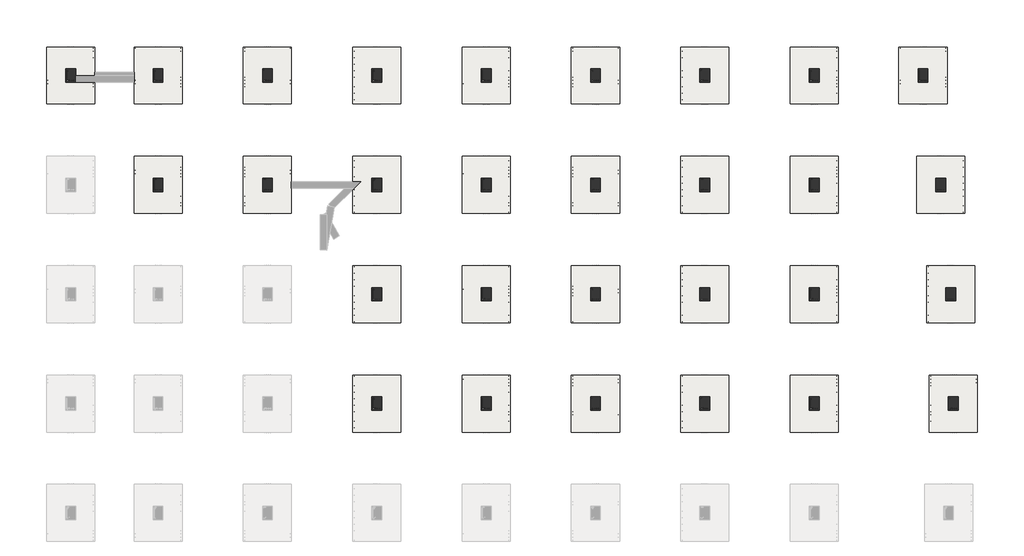
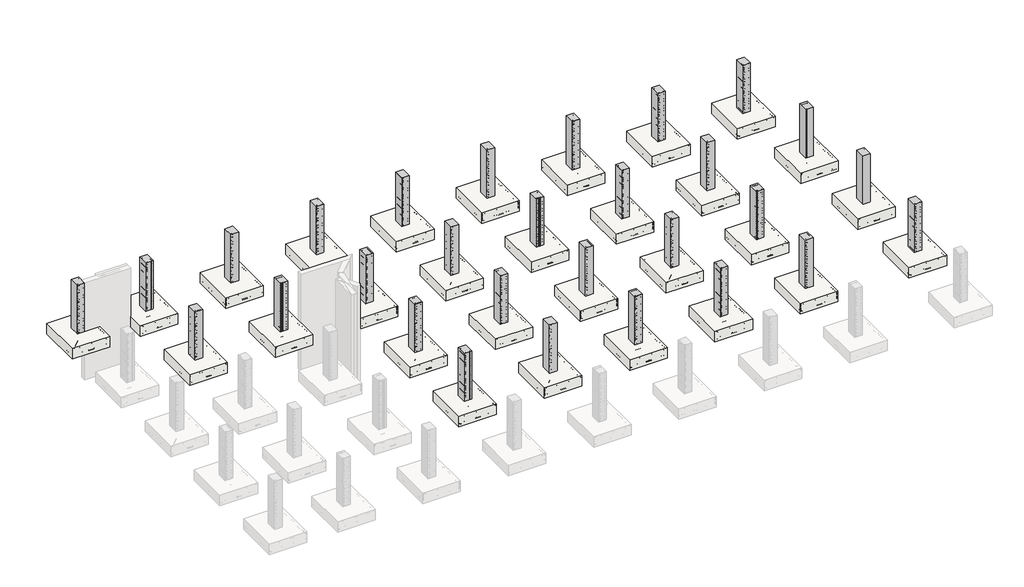
# One storey, part 2 of 33: 29 columns, 29 slabs.
"""IFC4 building model written with IfcOpenShell, lengths in millimetres."""

from ifc_helpers import new_model, si_unit, frame, origin, place, context, project, spatial, polyline, outline, extrude, element, save

model = new_model("IFC4")

# Units and contexts
model_context = context("Model", 3, world=origin())
ifc_project = project(units=[si_unit("LENGTHUNIT", "METRE", prefix="MILLI")], contexts=[model_context])

# Site, building, storey
site = spatial("IfcSite", under=ifc_project)
building = spatial("IfcBuilding", under=site)
storey = spatial("IfcBuildingStorey", under=building, Elevation=-3000.0)

# Columns
placement = place(None, origin())
element("IfcColumn", 1, ObjectType="M_Concrete-Rectangular-Column : 300 x 450mm", at=placement, inside=storey, context=model_context, shape_type="SweptSolid", body=[
    extrude(outline(polyline([(-13414.8142742, 17007.0891866), (-13414.8142742, 16397.4891866), (-13864.8142742, 16397.4891866), (-13864.8142742, 17007.0891866), (-13414.8142742, 17007.0891866)])), frame((0.0, 0.0, -3000.0), z_axis=(0.0, 0.0, 1.0), x_axis=(1.0, 0.0, 0.0)), (0.0, 0.0, 1.0), 3000.0),
])
element("IfcColumn", 2, ObjectType="M_Concrete-Rectangular-Column : 300 x 450mm", at=placement, inside=storey, context=model_context, shape_type="SweptSolid", body=[
    extrude(outline(polyline([(-9414.8142742, 17007.0891866), (-9414.8142742, 16397.4891866), (-9864.8142742, 16397.4891866), (-9864.8142742, 17007.0891866), (-9414.8142742, 17007.0891866)])), frame((0.0, 0.0, -3000.0), z_axis=(0.0, 0.0, 1.0), x_axis=(1.0, 0.0, 0.0)), (0.0, 0.0, 1.0), 3000.0),
])
element("IfcColumn", 3, ObjectType="M_Concrete-Rectangular-Column : 300 x 450mm", at=placement, inside=storey, context=model_context, shape_type="SweptSolid", body=[
    extrude(outline(polyline([(-9414.8142742, 12007.0891866), (-9414.8142742, 11397.4891866), (-9864.8142742, 11397.4891866), (-9864.8142742, 12007.0891866), (-9414.8142742, 12007.0891866)])), frame((0.0, 0.0, -3000.0), z_axis=(0.0, 0.0, 1.0), x_axis=(1.0, 0.0, 0.0)), (0.0, 0.0, 1.0), 3000.0),
])
element("IfcColumn", 4, ObjectType="M_Concrete-Rectangular-Column : 300 x 450mm", at=placement, inside=storey, context=model_context, shape_type="SweptSolid", body=[
    extrude(outline(polyline([(-4414.8142742, 17007.0891866), (-4414.8142742, 16397.4891866), (-4864.8142742, 16397.4891866), (-4864.8142742, 17007.0891866), (-4414.8142742, 17007.0891866)])), frame((0.0, 0.0, -3000.0), z_axis=(0.0, 0.0, 1.0), x_axis=(1.0, 0.0, 0.0)), (0.0, 0.0, 1.0), 3000.0),
])
element("IfcColumn", 5, ObjectType="M_Concrete-Rectangular-Column : 300 x 450mm", at=placement, inside=storey, context=model_context, shape_type="SweptSolid", body=[
    extrude(outline(polyline([(-4414.8142742, 12007.0891866), (-4414.8142742, 11397.4891866), (-4864.8142742, 11397.4891866), (-4864.8142742, 12007.0891866), (-4414.8142742, 12007.0891866)])), frame((0.0, 0.0, -3000.0), z_axis=(0.0, 0.0, 1.0), x_axis=(1.0, 0.0, 0.0)), (0.0, 0.0, 1.0), 3000.0),
])
element("IfcColumn", 6, ObjectType="M_Concrete-Rectangular-Column : 300 x 450mm", at=placement, inside=storey, context=model_context, shape_type="SweptSolid", body=[
    extrude(outline(polyline([(585.1857258, 17007.0891866), (585.1857258, 16397.4891866), (135.1857258, 16397.4891866), (135.1857258, 17007.0891866), (585.1857258, 17007.0891866)])), frame((0.0, 0.0, -3000.0), z_axis=(0.0, 0.0, 1.0), x_axis=(1.0, 0.0, 0.0)), (0.0, 0.0, 1.0), 3000.0),
])
element("IfcColumn", 7, ObjectType="M_Concrete-Rectangular-Column : 300 x 450mm", at=placement, inside=storey, context=model_context, shape_type="SweptSolid", body=[
    extrude(outline(polyline([(585.1857258, 12007.0891866), (585.1857258, 11397.4891866), (135.1857258, 11397.4891866), (135.1857258, 12007.0891866), (585.1857258, 12007.0891866)])), frame((0.0, 0.0, -3000.0), z_axis=(0.0, 0.0, 1.0), x_axis=(1.0, 0.0, 0.0)), (0.0, 0.0, 1.0), 3000.0),
])
element("IfcColumn", 8, ObjectType="M_Concrete-Rectangular-Column : 300 x 450mm", at=placement, inside=storey, context=model_context, shape_type="SweptSolid", body=[
    extrude(outline(polyline([(585.1857258, 7007.0891866), (585.1857258, 6397.4891866), (135.1857258, 6397.4891866), (135.1857258, 7007.0891866), (585.1857258, 7007.0891866)])), frame((0.0, 0.0, -3000.0), z_axis=(0.0, 0.0, 1.0), x_axis=(1.0, 0.0, 0.0)), (0.0, 0.0, 1.0), 3000.0),
])
element("IfcColumn", 9, ObjectType="M_Concrete-Rectangular-Column : 300 x 450mm", at=placement, inside=storey, context=model_context, shape_type="SweptSolid", body=[
    extrude(outline(polyline([(585.1857258, 2007.0891866), (585.1857258, 1397.4891866), (135.1857258, 1397.4891866), (135.1857258, 2007.0891866), (585.1857258, 2007.0891866)])), frame((0.0, 0.0, -3000.0), z_axis=(0.0, 0.0, 1.0), x_axis=(1.0, 0.0, 0.0)), (0.0, 0.0, 1.0), 3000.0),
])
element("IfcColumn", 10, ObjectType="M_Concrete-Rectangular-Column : 300 x 450mm", at=placement, inside=storey, context=model_context, shape_type="SweptSolid", body=[
    extrude(outline(polyline([(5585.1857258, 17007.0891866), (5585.1857258, 16397.4891866), (5135.1857258, 16397.4891866), (5135.1857258, 17007.0891866), (5585.1857258, 17007.0891866)])), frame((0.0, 0.0, -3000.0), z_axis=(0.0, 0.0, 1.0), x_axis=(1.0, 0.0, 0.0)), (0.0, 0.0, 1.0), 3000.0),
])
element("IfcColumn", 11, ObjectType="M_Concrete-Rectangular-Column : 300 x 450mm", at=placement, inside=storey, context=model_context, shape_type="SweptSolid", body=[
    extrude(outline(polyline([(5585.1857258, 12007.0891866), (5585.1857258, 11397.4891866), (5135.1857258, 11397.4891866), (5135.1857258, 12007.0891866), (5585.1857258, 12007.0891866)])), frame((0.0, 0.0, -3000.0), z_axis=(0.0, 0.0, 1.0), x_axis=(1.0, 0.0, 0.0)), (0.0, 0.0, 1.0), 3000.0),
])
element("IfcColumn", 12, ObjectType="M_Concrete-Rectangular-Column : 300 x 450mm", at=placement, inside=storey, context=model_context, shape_type="SweptSolid", body=[
    extrude(outline(polyline([(5585.1857258, 7007.0891866), (5585.1857258, 6397.4891866), (5135.1857258, 6397.4891866), (5135.1857258, 7007.0891866), (5585.1857258, 7007.0891866)])), frame((0.0, 0.0, -3000.0), z_axis=(0.0, 0.0, 1.0), x_axis=(1.0, 0.0, 0.0)), (0.0, 0.0, 1.0), 3000.0),
])
element("IfcColumn", 13, ObjectType="M_Concrete-Rectangular-Column : 300 x 450mm", at=placement, inside=storey, context=model_context, shape_type="SweptSolid", body=[
    extrude(outline(polyline([(5585.1857258, 2007.0891866), (5585.1857258, 1397.4891866), (5135.1857258, 1397.4891866), (5135.1857258, 2007.0891866), (5585.1857258, 2007.0891866)])), frame((0.0, 0.0, -3000.0), z_axis=(0.0, 0.0, 1.0), x_axis=(1.0, 0.0, 0.0)), (0.0, 0.0, 1.0), 3000.0),
])
element("IfcColumn", 14, ObjectType="M_Concrete-Rectangular-Column : 300 x 450mm", at=placement, inside=storey, context=model_context, shape_type="SweptSolid", body=[
    extrude(outline(polyline([(10585.1857258, 17007.0891866), (10585.1857258, 16397.4891866), (10135.1857258, 16397.4891866), (10135.1857258, 17007.0891866), (10585.1857258, 17007.0891866)])), frame((0.0, 0.0, -3000.0), z_axis=(0.0, 0.0, 1.0), x_axis=(1.0, 0.0, 0.0)), (0.0, 0.0, 1.0), 3000.0),
])
element("IfcColumn", 15, ObjectType="M_Concrete-Rectangular-Column : 300 x 450mm", at=placement, inside=storey, context=model_context, shape_type="SweptSolid", body=[
    extrude(outline(polyline([(10585.1857258, 12007.0891866), (10585.1857258, 11397.4891866), (10135.1857258, 11397.4891866), (10135.1857258, 12007.0891866), (10585.1857258, 12007.0891866)])), frame((0.0, 0.0, -3000.0), z_axis=(0.0, 0.0, 1.0), x_axis=(1.0, 0.0, 0.0)), (0.0, 0.0, 1.0), 3000.0),
])
element("IfcColumn", 16, ObjectType="M_Concrete-Rectangular-Column : 300 x 450mm", at=placement, inside=storey, context=model_context, shape_type="SweptSolid", body=[
    extrude(outline(polyline([(10585.1857258, 7007.0891866), (10585.1857258, 6397.4891866), (10135.1857258, 6397.4891866), (10135.1857258, 7007.0891866), (10585.1857258, 7007.0891866)])), frame((0.0, 0.0, -3000.0), z_axis=(0.0, 0.0, 1.0), x_axis=(1.0, 0.0, 0.0)), (0.0, 0.0, 1.0), 3000.0),
])
element("IfcColumn", 17, ObjectType="M_Concrete-Rectangular-Column : 300 x 450mm", at=placement, inside=storey, context=model_context, shape_type="SweptSolid", body=[
    extrude(outline(polyline([(10585.1857258, 2007.0891866), (10585.1857258, 1397.4891866), (10135.1857258, 1397.4891866), (10135.1857258, 2007.0891866), (10585.1857258, 2007.0891866)])), frame((0.0, 0.0, -3000.0), z_axis=(0.0, 0.0, 1.0), x_axis=(1.0, 0.0, 0.0)), (0.0, 0.0, 1.0), 3000.0),
])
element("IfcColumn", 18, ObjectType="M_Concrete-Rectangular-Column : 300 x 450mm", at=placement, inside=storey, context=model_context, shape_type="SweptSolid", body=[
    extrude(outline(polyline([(15585.1857258, 17007.0891866), (15585.1857258, 16397.4891866), (15135.1857258, 16397.4891866), (15135.1857258, 17007.0891866), (15585.1857258, 17007.0891866)])), frame((0.0, 0.0, -3000.0), z_axis=(0.0, 0.0, 1.0), x_axis=(1.0, 0.0, 0.0)), (0.0, 0.0, 1.0), 3000.0),
])
element("IfcColumn", 19, ObjectType="M_Concrete-Rectangular-Column : 300 x 450mm", at=placement, inside=storey, context=model_context, shape_type="SweptSolid", body=[
    extrude(outline(polyline([(15585.1857258, 12007.0891866), (15585.1857258, 11397.4891866), (15135.1857258, 11397.4891866), (15135.1857258, 12007.0891866), (15585.1857258, 12007.0891866)])), frame((0.0, 0.0, -3000.0), z_axis=(0.0, 0.0, 1.0), x_axis=(1.0, 0.0, 0.0)), (0.0, 0.0, 1.0), 3000.0),
])
element("IfcColumn", 20, ObjectType="M_Concrete-Rectangular-Column : 300 x 450mm", at=placement, inside=storey, context=model_context, shape_type="SweptSolid", body=[
    extrude(outline(polyline([(15585.1857258, 7007.0891866), (15585.1857258, 6397.4891866), (15135.1857258, 6397.4891866), (15135.1857258, 7007.0891866), (15585.1857258, 7007.0891866)])), frame((0.0, 0.0, -3000.0), z_axis=(0.0, 0.0, 1.0), x_axis=(1.0, 0.0, 0.0)), (0.0, 0.0, 1.0), 3000.0),
])
element("IfcColumn", 21, ObjectType="M_Concrete-Rectangular-Column : 300 x 450mm", at=placement, inside=storey, context=model_context, shape_type="SweptSolid", body=[
    extrude(outline(polyline([(15585.1857258, 2007.0891866), (15585.1857258, 1397.4891866), (15135.1857258, 1397.4891866), (15135.1857258, 2007.0891866), (15585.1857258, 2007.0891866)])), frame((0.0, 0.0, -3000.0), z_axis=(0.0, 0.0, 1.0), x_axis=(1.0, 0.0, 0.0)), (0.0, 0.0, 1.0), 3000.0),
])
element("IfcColumn", 22, ObjectType="M_Concrete-Rectangular-Column : 300 x 450mm", at=placement, inside=storey, context=model_context, shape_type="SweptSolid", body=[
    extrude(outline(polyline([(20585.1857258, 17007.0891866), (20585.1857258, 16397.4891866), (20135.1857258, 16397.4891866), (20135.1857258, 17007.0891866), (20585.1857258, 17007.0891866)])), frame((0.0, 0.0, -3000.0), z_axis=(0.0, 0.0, 1.0), x_axis=(1.0, 0.0, 0.0)), (0.0, 0.0, 1.0), 3000.0),
])
element("IfcColumn", 23, ObjectType="M_Concrete-Rectangular-Column : 300 x 450mm", at=placement, inside=storey, context=model_context, shape_type="SweptSolid", body=[
    extrude(outline(polyline([(20585.1857258, 12007.0891866), (20585.1857258, 11397.4891866), (20135.1857258, 11397.4891866), (20135.1857258, 12007.0891866), (20585.1857258, 12007.0891866)])), frame((0.0, 0.0, -3000.0), z_axis=(0.0, 0.0, 1.0), x_axis=(1.0, 0.0, 0.0)), (0.0, 0.0, 1.0), 3000.0),
])
element("IfcColumn", 24, ObjectType="M_Concrete-Rectangular-Column : 300 x 450mm", at=placement, inside=storey, context=model_context, shape_type="SweptSolid", body=[
    extrude(outline(polyline([(20585.1857258, 7007.0891866), (20585.1857258, 6397.4891866), (20135.1857258, 6397.4891866), (20135.1857258, 7007.0891866), (20585.1857258, 7007.0891866)])), frame((0.0, 0.0, -3000.0), z_axis=(0.0, 0.0, 1.0), x_axis=(1.0, 0.0, 0.0)), (0.0, 0.0, 1.0), 3000.0),
])
element("IfcColumn", 25, ObjectType="M_Concrete-Rectangular-Column : 300 x 450mm", at=placement, inside=storey, context=model_context, shape_type="SweptSolid", body=[
    extrude(outline(polyline([(20585.1857258, 2007.0891866), (20585.1857258, 1397.4891866), (20135.1857258, 1397.4891866), (20135.1857258, 2007.0891866), (20585.1857258, 2007.0891866)])), frame((0.0, 0.0, -3000.0), z_axis=(0.0, 0.0, 1.0), x_axis=(1.0, 0.0, 0.0)), (0.0, 0.0, 1.0), 3000.0),
])
element("IfcColumn", 26, ObjectType="M_Concrete-Rectangular-Column : 300 x 450mm", at=placement, inside=storey, context=model_context, shape_type="SweptSolid", body=[
    extrude(outline(polyline([(25564.5332373, 17007.0891866), (25564.5332373, 16397.4891866), (25114.5332373, 16397.4891866), (25114.5332373, 17007.0891866), (25564.5332373, 17007.0891866)])), frame((0.0, 0.0, -3000.0), z_axis=(0.0, 0.0, 1.0), x_axis=(1.0, 0.0, 0.0)), (0.0, 0.0, 1.0), 3000.0),
])
element("IfcColumn", 27, ObjectType="M_Concrete-Rectangular-Column : 300 x 450mm", at=placement, inside=storey, context=model_context, shape_type="SweptSolid", body=[
    extrude(outline(polyline([(26372.9223959, 12007.0891866), (26372.9223959, 11397.4891866), (25922.9223959, 11397.4891866), (25922.9223959, 12007.0891866), (26372.9223959, 12007.0891866)])), frame((0.0, 0.0, -3000.0), z_axis=(0.0, 0.0, 1.0), x_axis=(1.0, 0.0, 0.0)), (0.0, 0.0, 1.0), 3000.0),
])
element("IfcColumn", 28, ObjectType="M_Concrete-Rectangular-Column : 300 x 450mm", at=placement, inside=storey, context=model_context, shape_type="SweptSolid", body=[
    extrude(outline(polyline([(26833.3282195, 7007.0891866), (26833.3282195, 6397.4891866), (26383.3282195, 6397.4891866), (26383.3282195, 7007.0891866), (26833.3282195, 7007.0891866)])), frame((0.0, 0.0, -3000.0), z_axis=(0.0, 0.0, 1.0), x_axis=(1.0, 0.0, 0.0)), (0.0, 0.0, 1.0), 3000.0),
])
element("IfcColumn", 29, ObjectType="M_Concrete-Rectangular-Column : 300 x 450mm", at=placement, inside=storey, context=model_context, shape_type="SweptSolid", body=[
    extrude(outline(polyline([(26952.2756413, 2007.0891866), (26952.2756413, 1397.4891866), (26502.2756413, 1397.4891866), (26502.2756413, 2007.0891866), (26952.2756413, 2007.0891866)])), frame((0.0, 0.0, -3000.0), z_axis=(0.0, 0.0, 1.0), x_axis=(1.0, 0.0, 0.0)), (0.0, 0.0, 1.0), 3000.0),
])

# Slabs
element("IfcSlab", 30, ObjectType="M_Footing-Rectangular : 650X2200X2600", at=placement, inside=storey, context=model_context, shape_type="SweptSolid", body=[
    extrude(outline(polyline([(-12539.8142742, 18002.2891866), (-12539.8142742, 15402.2891866), (-14739.8142742, 15402.2891866), (-14739.8142742, 18002.2891866), (-12539.8142742, 18002.2891866)])), frame((0.0, 0.0, -3650.0), z_axis=(0.0, 0.0, 1.0), x_axis=(1.0, 0.0, 0.0)), (0.0, 0.0, 1.0), 650.0),
])
element("IfcSlab", 31, ObjectType="M_Footing-Rectangular : 650X2200X2600", at=placement, inside=storey, context=model_context, shape_type="SweptSolid", body=[
    extrude(outline(polyline([(-8539.8142742, 18002.2891866), (-8539.8142742, 15402.2891866), (-10739.8142742, 15402.2891866), (-10739.8142742, 18002.2891866), (-8539.8142742, 18002.2891866)])), frame((0.0, 0.0, -3650.0), z_axis=(0.0, 0.0, 1.0), x_axis=(1.0, 0.0, 0.0)), (0.0, 0.0, 1.0), 650.0),
])
element("IfcSlab", 32, ObjectType="M_Footing-Rectangular : 650X2200X2600", at=placement, inside=storey, context=model_context, shape_type="SweptSolid", body=[
    extrude(outline(polyline([(-8539.8142742, 13002.2891866), (-8539.8142742, 10402.2891866), (-10739.8142742, 10402.2891866), (-10739.8142742, 13002.2891866), (-8539.8142742, 13002.2891866)])), frame((0.0, 0.0, -3650.0), z_axis=(0.0, 0.0, 1.0), x_axis=(1.0, 0.0, 0.0)), (0.0, 0.0, 1.0), 650.0),
])
element("IfcSlab", 33, ObjectType="M_Footing-Rectangular : 650X2200X2600", at=placement, inside=storey, context=model_context, shape_type="SweptSolid", body=[
    extrude(outline(polyline([(-3539.8142742, 18002.2891866), (-3539.8142742, 15402.2891866), (-5739.8142742, 15402.2891866), (-5739.8142742, 18002.2891866), (-3539.8142742, 18002.2891866)])), frame((0.0, 0.0, -3650.0), z_axis=(0.0, 0.0, 1.0), x_axis=(1.0, 0.0, 0.0)), (0.0, 0.0, 1.0), 650.0),
])
element("IfcSlab", 34, ObjectType="M_Footing-Rectangular : 650X2200X2600", at=placement, inside=storey, context=model_context, shape_type="SweptSolid", body=[
    extrude(outline(polyline([(-3539.8142742, 13002.2891866), (-3539.8142742, 10402.2891866), (-5739.8142742, 10402.2891866), (-5739.8142742, 13002.2891866), (-3539.8142742, 13002.2891866)])), frame((0.0, 0.0, -3650.0), z_axis=(0.0, 0.0, 1.0), x_axis=(1.0, 0.0, 0.0)), (0.0, 0.0, 1.0), 650.0),
])
element("IfcSlab", 35, ObjectType="M_Footing-Rectangular : 650X2200X2600", at=placement, inside=storey, context=model_context, shape_type="SweptSolid", body=[
    extrude(outline(polyline([(1460.1857258, 18002.2891866), (1460.1857258, 15402.2891866), (-739.8142742, 15402.2891866), (-739.8142742, 18002.2891866), (1460.1857258, 18002.2891866)])), frame((0.0, 0.0, -3650.0), z_axis=(0.0, 0.0, 1.0), x_axis=(1.0, 0.0, 0.0)), (0.0, 0.0, 1.0), 650.0),
])
element("IfcSlab", 36, ObjectType="M_Footing-Rectangular : 650X2200X2600", at=placement, inside=storey, context=model_context, shape_type="SweptSolid", body=[
    extrude(outline(polyline([(1460.1857258, 13002.2891866), (1460.1857258, 10402.2891866), (-739.8142742, 10402.2891866), (-739.8142742, 13002.2891866), (1460.1857258, 13002.2891866)])), frame((0.0, 0.0, -3650.0), z_axis=(0.0, 0.0, 1.0), x_axis=(1.0, 0.0, 0.0)), (0.0, 0.0, 1.0), 650.0),
])
element("IfcSlab", 37, ObjectType="M_Footing-Rectangular : 650X2200X2600", at=placement, inside=storey, context=model_context, shape_type="SweptSolid", body=[
    extrude(outline(polyline([(1460.1857258, 8002.2891866), (1460.1857258, 5402.2891866), (-739.8142742, 5402.2891866), (-739.8142742, 8002.2891866), (1460.1857258, 8002.2891866)])), frame((0.0, 0.0, -3650.0), z_axis=(0.0, 0.0, 1.0), x_axis=(1.0, 0.0, 0.0)), (0.0, 0.0, 1.0), 650.0),
])
element("IfcSlab", 38, ObjectType="M_Footing-Rectangular : 650X2200X2600", at=placement, inside=storey, context=model_context, shape_type="SweptSolid", body=[
    extrude(outline(polyline([(1460.1857258, 3002.2891866), (1460.1857258, 402.2891866), (-739.8142742, 402.2891866), (-739.8142742, 3002.2891866), (1460.1857258, 3002.2891866)])), frame((0.0, 0.0, -3650.0), z_axis=(0.0, 0.0, 1.0), x_axis=(1.0, 0.0, 0.0)), (0.0, 0.0, 1.0), 650.0),
])
element("IfcSlab", 39, ObjectType="M_Footing-Rectangular : 650X2200X2600", at=placement, inside=storey, context=model_context, shape_type="SweptSolid", body=[
    extrude(outline(polyline([(6460.1857258, 18002.2891866), (6460.1857258, 15402.2891866), (4260.1857258, 15402.2891866), (4260.1857258, 18002.2891866), (6460.1857258, 18002.2891866)])), frame((0.0, 0.0, -3650.0), z_axis=(0.0, 0.0, 1.0), x_axis=(1.0, 0.0, 0.0)), (0.0, 0.0, 1.0), 650.0),
])
element("IfcSlab", 40, ObjectType="M_Footing-Rectangular : 650X2200X2600", at=placement, inside=storey, context=model_context, shape_type="SweptSolid", body=[
    extrude(outline(polyline([(6460.1857258, 13002.2891866), (6460.1857258, 10402.2891866), (4260.1857258, 10402.2891866), (4260.1857258, 13002.2891866), (6460.1857258, 13002.2891866)])), frame((0.0, 0.0, -3650.0), z_axis=(0.0, 0.0, 1.0), x_axis=(1.0, 0.0, 0.0)), (0.0, 0.0, 1.0), 650.0),
])
element("IfcSlab", 41, ObjectType="M_Footing-Rectangular : 650X2200X2600", at=placement, inside=storey, context=model_context, shape_type="SweptSolid", body=[
    extrude(outline(polyline([(6460.1857258, 8002.2891866), (6460.1857258, 5402.2891866), (4260.1857258, 5402.2891866), (4260.1857258, 8002.2891866), (6460.1857258, 8002.2891866)])), frame((0.0, 0.0, -3650.0), z_axis=(0.0, 0.0, 1.0), x_axis=(1.0, 0.0, 0.0)), (0.0, 0.0, 1.0), 650.0),
])
element("IfcSlab", 42, ObjectType="M_Footing-Rectangular : 650X2200X2600", at=placement, inside=storey, context=model_context, shape_type="SweptSolid", body=[
    extrude(outline(polyline([(6460.1857258, 3002.2891866), (6460.1857258, 402.2891866), (4260.1857258, 402.2891866), (4260.1857258, 3002.2891866), (6460.1857258, 3002.2891866)])), frame((0.0, 0.0, -3650.0), z_axis=(0.0, 0.0, 1.0), x_axis=(1.0, 0.0, 0.0)), (0.0, 0.0, 1.0), 650.0),
])
element("IfcSlab", 43, ObjectType="M_Footing-Rectangular : 650X2200X2600", at=placement, inside=storey, context=model_context, shape_type="SweptSolid", body=[
    extrude(outline(polyline([(11460.1857258, 18002.2891866), (11460.1857258, 15402.2891866), (9260.1857258, 15402.2891866), (9260.1857258, 18002.2891866), (11460.1857258, 18002.2891866)])), frame((0.0, 0.0, -3650.0), z_axis=(0.0, 0.0, 1.0), x_axis=(1.0, 0.0, 0.0)), (0.0, 0.0, 1.0), 650.0),
])
element("IfcSlab", 44, ObjectType="M_Footing-Rectangular : 650X2200X2600", at=placement, inside=storey, context=model_context, shape_type="SweptSolid", body=[
    extrude(outline(polyline([(11460.1857258, 13002.2891866), (11460.1857258, 10402.2891866), (9260.1857258, 10402.2891866), (9260.1857258, 13002.2891866), (11460.1857258, 13002.2891866)])), frame((0.0, 0.0, -3650.0), z_axis=(0.0, 0.0, 1.0), x_axis=(1.0, 0.0, 0.0)), (0.0, 0.0, 1.0), 650.0),
])
element("IfcSlab", 45, ObjectType="M_Footing-Rectangular : 650X2200X2600", at=placement, inside=storey, context=model_context, shape_type="SweptSolid", body=[
    extrude(outline(polyline([(11460.1857258, 8002.2891866), (11460.1857258, 5402.2891866), (9260.1857258, 5402.2891866), (9260.1857258, 8002.2891866), (11460.1857258, 8002.2891866)])), frame((0.0, 0.0, -3650.0), z_axis=(0.0, 0.0, 1.0), x_axis=(1.0, 0.0, 0.0)), (0.0, 0.0, 1.0), 650.0),
])
element("IfcSlab", 46, ObjectType="M_Footing-Rectangular : 650X2200X2600", at=placement, inside=storey, context=model_context, shape_type="SweptSolid", body=[
    extrude(outline(polyline([(11460.1857258, 3002.2891866), (11460.1857258, 402.2891866), (9260.1857258, 402.2891866), (9260.1857258, 3002.2891866), (11460.1857258, 3002.2891866)])), frame((0.0, 0.0, -3650.0), z_axis=(0.0, 0.0, 1.0), x_axis=(1.0, 0.0, 0.0)), (0.0, 0.0, 1.0), 650.0),
])
element("IfcSlab", 47, ObjectType="M_Footing-Rectangular : 650X2200X2600", at=placement, inside=storey, context=model_context, shape_type="SweptSolid", body=[
    extrude(outline(polyline([(16460.1857258, 18002.2891866), (16460.1857258, 15402.2891866), (14260.1857258, 15402.2891866), (14260.1857258, 18002.2891866), (16460.1857258, 18002.2891866)])), frame((0.0, 0.0, -3650.0), z_axis=(0.0, 0.0, 1.0), x_axis=(1.0, 0.0, 0.0)), (0.0, 0.0, 1.0), 650.0),
])
element("IfcSlab", 48, ObjectType="M_Footing-Rectangular : 650X2200X2600", at=placement, inside=storey, context=model_context, shape_type="SweptSolid", body=[
    extrude(outline(polyline([(16460.1857258, 13002.2891866), (16460.1857258, 10402.2891866), (14260.1857258, 10402.2891866), (14260.1857258, 13002.2891866), (16460.1857258, 13002.2891866)])), frame((0.0, 0.0, -3650.0), z_axis=(0.0, 0.0, 1.0), x_axis=(1.0, 0.0, 0.0)), (0.0, 0.0, 1.0), 650.0),
])
element("IfcSlab", 49, ObjectType="M_Footing-Rectangular : 650X2200X2600", at=placement, inside=storey, context=model_context, shape_type="SweptSolid", body=[
    extrude(outline(polyline([(16460.1857258, 8002.2891866), (16460.1857258, 5402.2891866), (14260.1857258, 5402.2891866), (14260.1857258, 8002.2891866), (16460.1857258, 8002.2891866)])), frame((0.0, 0.0, -3650.0), z_axis=(0.0, 0.0, 1.0), x_axis=(1.0, 0.0, 0.0)), (0.0, 0.0, 1.0), 650.0),
])
element("IfcSlab", 50, ObjectType="M_Footing-Rectangular : 650X2200X2600", at=placement, inside=storey, context=model_context, shape_type="SweptSolid", body=[
    extrude(outline(polyline([(16460.1857258, 3002.2891866), (16460.1857258, 402.2891866), (14260.1857258, 402.2891866), (14260.1857258, 3002.2891866), (16460.1857258, 3002.2891866)])), frame((0.0, 0.0, -3650.0), z_axis=(0.0, 0.0, 1.0), x_axis=(1.0, 0.0, 0.0)), (0.0, 0.0, 1.0), 650.0),
])
element("IfcSlab", 51, ObjectType="M_Footing-Rectangular : 650X2200X2600", at=placement, inside=storey, context=model_context, shape_type="SweptSolid", body=[
    extrude(outline(polyline([(21460.1857258, 18002.2891866), (21460.1857258, 15402.2891866), (19260.1857258, 15402.2891866), (19260.1857258, 18002.2891866), (21460.1857258, 18002.2891866)])), frame((0.0, 0.0, -3650.0), z_axis=(0.0, 0.0, 1.0), x_axis=(1.0, 0.0, 0.0)), (0.0, 0.0, 1.0), 650.0),
])
element("IfcSlab", 52, ObjectType="M_Footing-Rectangular : 650X2200X2600", at=placement, inside=storey, context=model_context, shape_type="SweptSolid", body=[
    extrude(outline(polyline([(21460.1857258, 13002.2891866), (21460.1857258, 10402.2891866), (19260.1857258, 10402.2891866), (19260.1857258, 13002.2891866), (21460.1857258, 13002.2891866)])), frame((0.0, 0.0, -3650.0), z_axis=(0.0, 0.0, 1.0), x_axis=(1.0, 0.0, 0.0)), (0.0, 0.0, 1.0), 650.0),
])
element("IfcSlab", 53, ObjectType="M_Footing-Rectangular : 650X2200X2600", at=placement, inside=storey, context=model_context, shape_type="SweptSolid", body=[
    extrude(outline(polyline([(21460.1857258, 8002.2891866), (21460.1857258, 5402.2891866), (19260.1857258, 5402.2891866), (19260.1857258, 8002.2891866), (21460.1857258, 8002.2891866)])), frame((0.0, 0.0, -3650.0), z_axis=(0.0, 0.0, 1.0), x_axis=(1.0, 0.0, 0.0)), (0.0, 0.0, 1.0), 650.0),
])
element("IfcSlab", 54, ObjectType="M_Footing-Rectangular : 650X2200X2600", at=placement, inside=storey, context=model_context, shape_type="SweptSolid", body=[
    extrude(outline(polyline([(21460.1857258, 3002.2891866), (21460.1857258, 402.2891866), (19260.1857258, 402.2891866), (19260.1857258, 3002.2891866), (21460.1857258, 3002.2891866)])), frame((0.0, 0.0, -3650.0), z_axis=(0.0, 0.0, 1.0), x_axis=(1.0, 0.0, 0.0)), (0.0, 0.0, 1.0), 650.0),
])
element("IfcSlab", 55, ObjectType="M_Footing-Rectangular : 650X2200X2600", at=placement, inside=storey, context=model_context, shape_type="SweptSolid", body=[
    extrude(outline(polyline([(26439.5332373, 18002.2891866), (26439.5332373, 15402.2891866), (24239.5332373, 15402.2891866), (24239.5332373, 18002.2891866), (26439.5332373, 18002.2891866)])), frame((0.0, 0.0, -3650.0), z_axis=(0.0, 0.0, 1.0), x_axis=(1.0, 0.0, 0.0)), (0.0, 0.0, 1.0), 650.0),
])
element("IfcSlab", 56, ObjectType="M_Footing-Rectangular : 650X2200X2600", at=placement, inside=storey, context=model_context, shape_type="SweptSolid", body=[
    extrude(outline(polyline([(27247.9223959, 13002.2891866), (27247.9223959, 10402.2891866), (25047.9223959, 10402.2891866), (25047.9223959, 13002.2891866), (27247.9223959, 13002.2891866)])), frame((0.0, 0.0, -3650.0), z_axis=(0.0, 0.0, 1.0), x_axis=(1.0, 0.0, 0.0)), (0.0, 0.0, 1.0), 650.0),
])
element("IfcSlab", 57, ObjectType="M_Footing-Rectangular : 650X2200X2600", at=placement, inside=storey, context=model_context, shape_type="SweptSolid", body=[
    extrude(outline(polyline([(27708.3282195, 8002.2891866), (27708.3282195, 5402.2891866), (25508.3282195, 5402.2891866), (25508.3282195, 8002.2891866), (27708.3282195, 8002.2891866)])), frame((0.0, 0.0, -3650.0), z_axis=(0.0, 0.0, 1.0), x_axis=(1.0, 0.0, 0.0)), (0.0, 0.0, 1.0), 650.0),
])
element("IfcSlab", 58, ObjectType="M_Footing-Rectangular : 650X2200X2600", at=placement, inside=storey, context=model_context, shape_type="SweptSolid", body=[
    extrude(outline(polyline([(27827.2756413, 3002.2891866), (27827.2756413, 402.2891866), (25627.2756413, 402.2891866), (25627.2756413, 3002.2891866), (27827.2756413, 3002.2891866)])), frame((0.0, 0.0, -3650.0), z_axis=(0.0, 0.0, 1.0), x_axis=(1.0, 0.0, 0.0)), (0.0, 0.0, 1.0), 650.0),
])

save(model, "model.ifc")

# Revit data of these elements
# Type "M_Concrete-Rectangular-Column : 300 x 450mm"
#   b = 450 mm
#   h = 609.6 mm
#   Structural Material [instance default] = Concrete, Cast-in-Place gray
# Type "M_Footing-Rectangular : 650X2200X2600"
#   Width = 2200 mm
#   Length = 2600 mm
#   Foundation Thickness = 650 mm
#   Structural Material [instance default] = Concrete, Cast-in-Place gray
#   Assembly Code = ""
# Elements 1, 2, 3, 4, 5, 6, 7, 8, 9, 10, 11, 12, 13, 14, 15, 16, 17, 18, 19, 20, 21, 22, 23, 24, 25, 26, 27, 28, 29 (IfcColumn, "M_Concrete-Rectangular-Column : 300 x 450mm")
#   Structural Material = Default New Material
#   Phase Created = New Construction
#   Materials on its faces: "Default New Material"
# Elements 30, 31, 32, 33, 34, 35, 36, 37, 38, 39, 40, 41, 42, 43, 44, 45, 46, 47, 48, 49, 50, 51, 52, 53, 54, 55, 56, 57, 58 (IfcSlab, "M_Footing-Rectangular : 650X2200X2600")
#   Structural Material = Concrete, Cast-in-Place gray
#   Phase Created = New Construction
#   Materials on its faces: "Concrete, Cast-in-Place gray"
# Materials
#   "Concrete, Cast-in-Place gray": class "Concrete", colour RGB 130 132 119, transparency 0, Description = "Cast-in-place concrete", Cost = 0
#   "Default New Material": class "Generic", colour RGB 184 184 178, transparency 0, Cost = 0
